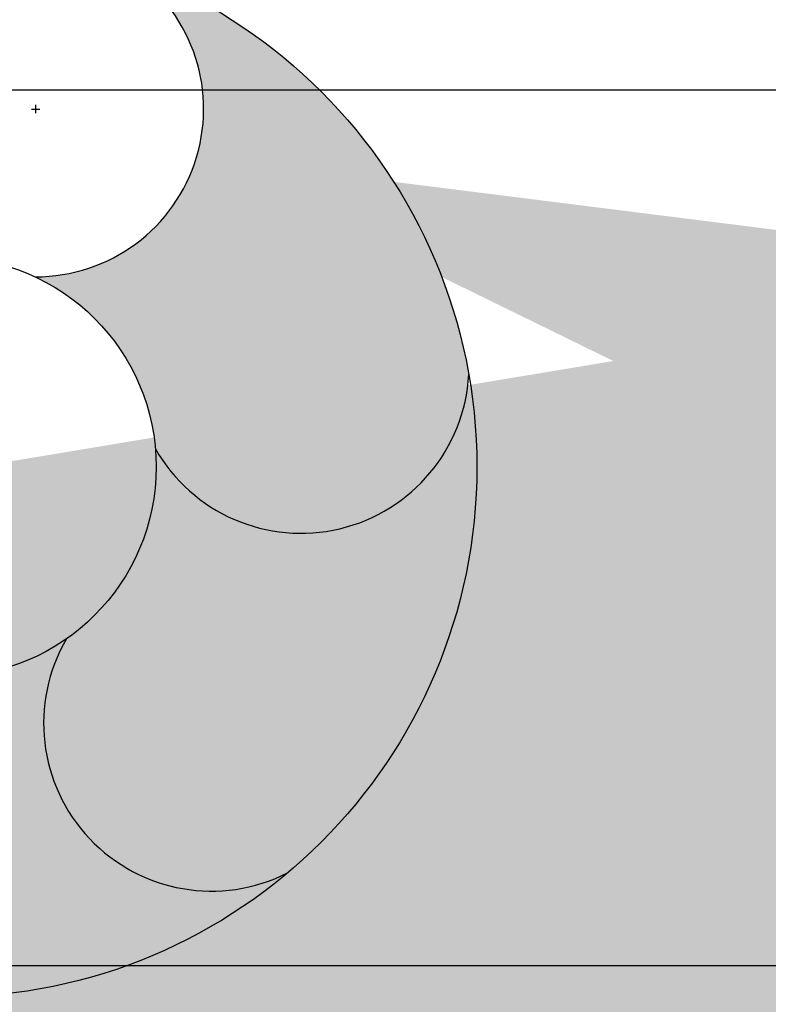
# Model space of a CAD drawing. Units: millimetres. Extents: x -22994 to 29398, y -19990 to 20176.
# Tile 117 of 135: x 229 to 245, y 135 to 156. Entities that reach past the tile are written whole.
import ezdxf

# ---------------------------------------------------------------- set-up
doc = ezdxf.new("R2010")
doc.units = ezdxf.units.MM
doc.header["$MEASUREMENT"] = 0
for name, color, linetype, lineweight in [('M-DIMS', 2, 'Continuous', 18), ('M-EQPM', 7, 'Continuous', 25), ('M-EQPM-PATT', 7, 'Continuous', 18)]:
    doc.layers.add(name, color=color, linetype=linetype, lineweight=lineweight)
doc.styles.get("Standard").update_dxf_attribs({"font": 'arial.ttf'})
doc.dimstyles.get("Standard").update_dxf_attribs({"dimtxt": 0.18, "dimasz": 10000, "dimexe": 0.18, "dimexo": 0.0625, "dimgap": 0.09, "dimtad": 0, "dimtih": 1, "dimtoh": 1, "dimdec": 0, "dimzin": 0, "dimdsep": 46, "dimtxsty": 'Standard', "dimcen": 0.09, "dimadec": 0, "dimazin": 0, "dimtfac": 1, "dimtdec": 0, "dimtofl": 0, "dimtmove": 0, "dimatfit": 3, "dimfxl": 1, "dimtolj": 1, "dimtzin": 0, "dimlwd": 30, "dimarcsym": 0})

# ---------------------------------------------------------------- blocks, each defined once
blk = doc.blocks.new('*D2')
at = {"layer": 'Defpoints', "color": 0, "transparency": 16777216}
for p in [(6.677, 10.271), (290.852, 10.271), (290.852, -5.079)]:
    blk.add_point(p, dxfattribs=at)
at = {"layer": 'M-DIMS', "color": 0, "lineweight": -2, "transparency": 16777216}
for p, q in [((6.677, 10.209), (6.677, -5.259)), ((290.852, 10.209), (290.852, -5.259))]:
    blk.add_line(p, q, dxfattribs=at)
at = {"layer": 'M-DIMS', "color": 0, "lineweight": 30, "transparency": 16777216}
for p, q in [((-9993.323, -5.079), (-19993.323, -5.079)), ((10290.852, -5.079), (20290.852, -5.079))]:
    blk.add_line(p, q, dxfattribs=at)
at = {"layer": 'M-DIMS', "color": 0, "transparency": 16777216}
for points in [[(-9993.323, 1661.588), (-9993.323, -1671.745), (6.677, -5.079)], [(10290.852, 1661.588), (10290.852, -1671.745), (290.852, -5.079)]]:
    blk.add_solid(points, dxfattribs=at)
at = {"layer": 'M-DIMS', "color": 0, "transparency": 16777216, "insert": (148.765, -5.079), "char_height": 0.18, "attachment_point": 5}
blk.add_mtext('\\A1;284.2', dxfattribs=at)
blk = doc.blocks.new('*D3')
at = {"layer": 'Defpoints', "color": 0, "transparency": 16777216}
for p in [(110.265, 204.165), (110.265, 176.366), (95.833, 127.967)]:
    blk.add_point(p, dxfattribs=at)
at = {"layer": 'M-DIMS', "color": 0, "lineweight": -2, "transparency": 16777216}
for p, q in [((95.833, 128.03), (95.833, 204.345)), ((110.265, 176.429), (110.265, 204.345))]:
    blk.add_line(p, q, dxfattribs=at)
at = {"layer": 'M-DIMS', "color": 0, "lineweight": 30, "transparency": 16777216}
for p, q in [((-9904.167, 204.165), (-19904.167, 204.165)), ((10110.265, 204.165), (20110.265, 204.165))]:
    blk.add_line(p, q, dxfattribs=at)
at = {"layer": 'M-DIMS', "color": 0, "transparency": 16777216}
for points in [[(-9904.167, 1870.832), (-9904.167, -1462.501), (95.833, 204.165)], [(10110.265, 1870.832), (10110.265, -1462.501), (110.265, 204.165)]]:
    blk.add_solid(points, dxfattribs=at)
at = {"layer": 'M-DIMS', "color": 0, "transparency": 16777216, "insert": (103.049, 204.165), "char_height": 0.18, "attachment_point": 5}
blk.add_mtext('\\A1;14.432', dxfattribs=at)
blk = doc.blocks.new('*D4')
at = {"layer": 'Defpoints', "color": 0, "transparency": 16777216}
for p in [(116.265, 204.165), (110.265, 176.366), (116.265, 176.366)]:
    blk.add_point(p, dxfattribs=at)
at = {"layer": 'M-DIMS', "color": 0, "lineweight": -2, "transparency": 16777216}
for p, q in [((110.265, 176.429), (110.265, 204.345)), ((116.265, 176.429), (116.265, 204.345))]:
    blk.add_line(p, q, dxfattribs=at)
at = {"layer": 'M-DIMS', "color": 0, "lineweight": 30, "transparency": 16777216}
for p, q in [((-9889.735, 204.165), (-19889.735, 204.165)), ((10116.265, 204.165), (20116.265, 204.165))]:
    blk.add_line(p, q, dxfattribs=at)
at = {"layer": 'M-DIMS', "color": 0, "transparency": 16777216}
for points in [[(-9889.735, 1870.832), (-9889.735, -1462.501), (110.265, 204.165)], [(10116.265, 1870.832), (10116.265, -1462.501), (116.265, 204.165)]]:
    blk.add_solid(points, dxfattribs=at)
at = {"layer": 'M-DIMS', "color": 0, "transparency": 16777216, "insert": (113.265, 204.165), "char_height": 0.18, "attachment_point": 5}
blk.add_mtext('\\A1;6', dxfattribs=at)
blk = doc.blocks.new('*D5')
at = {"layer": 'Defpoints', "color": 0, "transparency": 16777216}
for p in [(181.265, 204.165), (116.265, 176.366), (181.265, 176.366)]:
    blk.add_point(p, dxfattribs=at)
at = {"layer": 'M-DIMS', "color": 0, "lineweight": -2, "transparency": 16777216}
for p, q in [((116.265, 176.429), (116.265, 204.345)), ((181.265, 176.429), (181.265, 204.345))]:
    blk.add_line(p, q, dxfattribs=at)
at = {"layer": 'M-DIMS', "color": 0, "lineweight": 30, "transparency": 16777216}
for p, q in [((-9883.735, 204.165), (-19883.735, 204.165)), ((10181.265, 204.165), (20181.265, 204.165))]:
    blk.add_line(p, q, dxfattribs=at)
at = {"layer": 'M-DIMS', "color": 0, "transparency": 16777216}
for points in [[(-9883.735, 1870.832), (-9883.735, -1462.501), (116.265, 204.165)], [(10181.265, 1870.832), (10181.265, -1462.501), (181.265, 204.165)]]:
    blk.add_solid(points, dxfattribs=at)
at = {"layer": 'M-DIMS', "color": 0, "transparency": 16777216, "insert": (148.765, 204.165), "char_height": 0.18, "attachment_point": 5}
blk.add_mtext('\\A1;65', dxfattribs=at)
blk = doc.blocks.new('*D6')
at = {"layer": 'Defpoints', "color": 0, "transparency": 16777216}
for p in [(187.265, 204.165), (181.265, 176.366), (187.265, 176.366)]:
    blk.add_point(p, dxfattribs=at)
at = {"layer": 'M-DIMS', "color": 0, "lineweight": -2, "transparency": 16777216}
for p, q in [((181.265, 176.429), (181.265, 204.345)), ((187.265, 176.429), (187.265, 204.345))]:
    blk.add_line(p, q, dxfattribs=at)
at = {"layer": 'M-DIMS', "color": 0, "lineweight": 30, "transparency": 16777216}
for p, q in [((-9818.735, 204.165), (-19818.735, 204.165)), ((10187.265, 204.165), (20187.265, 204.165))]:
    blk.add_line(p, q, dxfattribs=at)
at = {"layer": 'M-DIMS', "color": 0, "transparency": 16777216}
for points in [[(-9818.735, 1870.832), (-9818.735, -1462.501), (181.265, 204.165)], [(10187.265, 1870.832), (10187.265, -1462.501), (187.265, 204.165)]]:
    blk.add_solid(points, dxfattribs=at)
at = {"layer": 'M-DIMS', "color": 0, "transparency": 16777216, "insert": (184.265, 204.165), "char_height": 0.18, "attachment_point": 5}
blk.add_mtext('\\A1;6', dxfattribs=at)
blk = doc.blocks.new('*D7')
at = {"layer": 'Defpoints', "color": 0, "transparency": 16777216}
for p in [(201.697, 204.165), (187.265, 176.366), (201.697, 127.967)]:
    blk.add_point(p, dxfattribs=at)
at = {"layer": 'M-DIMS', "color": 0, "lineweight": -2, "transparency": 16777216}
for p, q in [((187.265, 176.429), (187.265, 204.345)), ((201.697, 128.03), (201.697, 204.345))]:
    blk.add_line(p, q, dxfattribs=at)
at = {"layer": 'M-DIMS', "color": 0, "lineweight": 30, "transparency": 16777216}
for p, q in [((-9812.735, 204.165), (-19812.735, 204.165)), ((10201.697, 204.165), (20201.697, 204.165))]:
    blk.add_line(p, q, dxfattribs=at)
at = {"layer": 'M-DIMS', "color": 0, "transparency": 16777216}
for points in [[(-9812.735, 1870.832), (-9812.735, -1462.501), (187.265, 204.165)], [(10201.697, 1870.832), (10201.697, -1462.501), (201.697, 204.165)]]:
    blk.add_solid(points, dxfattribs=at)
at = {"layer": 'M-DIMS', "color": 0, "transparency": 16777216, "insert": (194.481, 204.165), "char_height": 0.18, "attachment_point": 5}
blk.add_mtext('\\A1;14.432', dxfattribs=at)
blk = doc.blocks.new('*D8')
at = {"layer": 'Defpoints', "color": 0, "transparency": 16777216}
for p in [(227.648, 204.165), (227.648, 146.73), (201.697, 127.967)]:
    blk.add_point(p, dxfattribs=at)
at = {"layer": 'M-DIMS', "color": 0, "lineweight": -2, "transparency": 16777216}
for p, q in [((201.697, 128.03), (201.697, 204.345)), ((227.648, 146.792), (227.648, 204.345))]:
    blk.add_line(p, q, dxfattribs=at)
at = {"layer": 'M-DIMS', "color": 0, "lineweight": 30, "transparency": 16777216}
for p, q in [((-9798.303, 204.165), (-19798.303, 204.165)), ((10227.648, 204.165), (20227.648, 204.165))]:
    blk.add_line(p, q, dxfattribs=at)
at = {"layer": 'M-DIMS', "color": 0, "transparency": 16777216}
for points in [[(-9798.303, 1870.832), (-9798.303, -1462.501), (201.697, 204.165)], [(10227.648, 1870.832), (10227.648, -1462.501), (227.648, 204.165)]]:
    blk.add_solid(points, dxfattribs=at)
at = {"layer": 'M-DIMS', "color": 0, "transparency": 16777216, "insert": (214.673, 204.165), "char_height": 0.18, "attachment_point": 5}
blk.add_mtext('\\A1;25.95', dxfattribs=at)
blk = doc.blocks.new('*D9')
at = {"layer": 'Defpoints', "color": 0, "transparency": 16777216}
for p in [(187.265, 176.366), (306.202, 176.366), (290.852, 10.271)]:
    blk.add_point(p, dxfattribs=at)
at = {"layer": 'M-DIMS', "color": 0, "lineweight": 30, "transparency": 16777216}
for p, q in [((306.202, 10176.366), (306.202, 20176.366)), ((306.202, -9989.729), (306.202, -19989.729))]:
    blk.add_line(p, q, dxfattribs=at)
at = {"layer": 'M-DIMS', "color": 0, "lineweight": -2, "transparency": 16777216}
for p, q in [((187.327, 176.366), (306.382, 176.366)), ((290.915, 10.271), (306.382, 10.271))]:
    blk.add_line(p, q, dxfattribs=at)
at = {"layer": 'M-DIMS', "color": 0, "transparency": 16777216}
for points in [[(-1360.465, 10176.366), (1972.869, 10176.366), (306.202, 176.366)], [(-1360.465, -9989.729), (1972.869, -9989.729), (306.202, 10.271)]]:
    blk.add_solid(points, dxfattribs=at)
at = {"layer": 'M-DIMS', "color": 0, "transparency": 16777216, "insert": (306.202, 93.319), "char_height": 0.18, "attachment_point": 5}
blk.add_mtext('\\A1;166.1', dxfattribs=at)
blk = doc.blocks.new('*D10')
at = {"layer": 'Defpoints', "color": 0, "transparency": 16777216}
for p in [(125.65, 136.071), (133.346, 136.071), (133.346, -5.079)]:
    blk.add_point(p, dxfattribs=at)
at = {"layer": 'M-DIMS', "color": 0, "lineweight": -2, "transparency": 16777216}
for p, q in [((125.65, 136.009), (125.65, -5.259)), ((133.346, 136.009), (133.346, -5.259))]:
    blk.add_line(p, q, dxfattribs=at)
at = {"layer": 'M-DIMS', "color": 0, "lineweight": 30, "transparency": 16777216}
for p, q in [((-9874.35, -5.079), (-19874.35, -5.079)), ((10133.346, -5.079), (20133.346, -5.079))]:
    blk.add_line(p, q, dxfattribs=at)
at = {"layer": 'M-DIMS', "color": 0, "transparency": 16777216}
for points in [[(-9874.35, 1661.588), (-9874.35, -1671.745), (125.65, -5.079)], [(10133.346, 1661.588), (10133.346, -1671.745), (133.346, -5.079)]]:
    blk.add_solid(points, dxfattribs=at)
at = {"layer": 'M-DIMS', "color": 0, "transparency": 16777216, "insert": (129.498, -5.079), "char_height": 0.18, "attachment_point": 5}
blk.add_mtext('\\A1;7.696', dxfattribs=at)
blk = doc.blocks.new('*D11')
at = {"layer": 'Defpoints', "color": 0, "transparency": 16777216}
for p in [(133.346, 136.071), (135.65, 136.071), (135.65, -5.079)]:
    blk.add_point(p, dxfattribs=at)
at = {"layer": 'M-DIMS', "color": 0, "lineweight": -2, "transparency": 16777216}
for p, q in [((133.346, 136.009), (133.346, -5.259)), ((135.65, 136.009), (135.65, -5.259))]:
    blk.add_line(p, q, dxfattribs=at)
at = {"layer": 'M-DIMS', "color": 0, "lineweight": 30, "transparency": 16777216}
for p, q in [((-9866.654, -5.079), (-19866.654, -5.079)), ((10135.65, -5.079), (20135.65, -5.079))]:
    blk.add_line(p, q, dxfattribs=at)
at = {"layer": 'M-DIMS', "color": 0, "transparency": 16777216}
for points in [[(-9866.654, 1661.588), (-9866.654, -1671.745), (133.346, -5.079)], [(10135.65, 1661.588), (10135.65, -1671.745), (135.65, -5.079)]]:
    blk.add_solid(points, dxfattribs=at)
at = {"layer": 'M-DIMS', "color": 0, "transparency": 16777216, "insert": (134.498, -5.079), "char_height": 0.18, "attachment_point": 5}
blk.add_mtext('\\A1;2.304', dxfattribs=at)
blk = doc.blocks.new('*D12')
at = {"layer": 'Defpoints', "color": 0, "transparency": 16777216}
for p in [(135.65, 136.071), (145.65, 136.071), (145.65, -5.079)]:
    blk.add_point(p, dxfattribs=at)
at = {"layer": 'M-DIMS', "color": 0, "lineweight": -2, "transparency": 16777216}
for p, q in [((135.65, 136.009), (135.65, -5.259)), ((145.65, 136.009), (145.65, -5.259))]:
    blk.add_line(p, q, dxfattribs=at)
at = {"layer": 'M-DIMS', "color": 0, "lineweight": 30, "transparency": 16777216}
for p, q in [((-9864.35, -5.079), (-19864.35, -5.079)), ((10145.65, -5.079), (20145.65, -5.079))]:
    blk.add_line(p, q, dxfattribs=at)
at = {"layer": 'M-DIMS', "color": 0, "transparency": 16777216}
for points in [[(-9864.35, 1661.588), (-9864.35, -1671.745), (135.65, -5.079)], [(10145.65, 1661.588), (10145.65, -1671.745), (145.65, -5.079)]]:
    blk.add_solid(points, dxfattribs=at)
at = {"layer": 'M-DIMS', "color": 0, "transparency": 16777216, "insert": (140.65, -5.079), "char_height": 0.18, "attachment_point": 5}
blk.add_mtext('\\A1;10', dxfattribs=at)
blk = doc.blocks.new('*D13')
at = {"layer": 'Defpoints', "color": 0, "transparency": 16777216}
for p in [(145.65, 136.071), (155.65, 136.071), (155.65, -5.079)]:
    blk.add_point(p, dxfattribs=at)
at = {"layer": 'M-DIMS', "color": 0, "lineweight": -2, "transparency": 16777216}
for p, q in [((145.65, 136.009), (145.65, -5.259)), ((155.65, 136.009), (155.65, -5.259))]:
    blk.add_line(p, q, dxfattribs=at)
at = {"layer": 'M-DIMS', "color": 0, "lineweight": 30, "transparency": 16777216}
for p, q in [((-9854.35, -5.079), (-19854.35, -5.079)), ((10155.65, -5.079), (20155.65, -5.079))]:
    blk.add_line(p, q, dxfattribs=at)
at = {"layer": 'M-DIMS', "color": 0, "transparency": 16777216}
for points in [[(-9854.35, 1661.588), (-9854.35, -1671.745), (145.65, -5.079)], [(10155.65, 1661.588), (10155.65, -1671.745), (155.65, -5.079)]]:
    blk.add_solid(points, dxfattribs=at)
at = {"layer": 'M-DIMS', "color": 0, "transparency": 16777216, "insert": (150.65, -5.079), "char_height": 0.18, "attachment_point": 5}
blk.add_mtext('\\A1;10', dxfattribs=at)
blk = doc.blocks.new('*D14')
at = {"layer": 'Defpoints', "color": 0, "transparency": 16777216}
for p in [(155.65, 136.071), (165.65, 136.071), (165.65, -5.079)]:
    blk.add_point(p, dxfattribs=at)
at = {"layer": 'M-DIMS', "color": 0, "lineweight": -2, "transparency": 16777216}
for p, q in [((155.65, 136.009), (155.65, -5.259)), ((165.65, 136.009), (165.65, -5.259))]:
    blk.add_line(p, q, dxfattribs=at)
at = {"layer": 'M-DIMS', "color": 0, "lineweight": 30, "transparency": 16777216}
for p, q in [((-9844.35, -5.079), (-19844.35, -5.079)), ((10165.65, -5.079), (20165.65, -5.079))]:
    blk.add_line(p, q, dxfattribs=at)
at = {"layer": 'M-DIMS', "color": 0, "transparency": 16777216}
for points in [[(-9844.35, 1661.588), (-9844.35, -1671.745), (155.65, -5.079)], [(10165.65, 1661.588), (10165.65, -1671.745), (165.65, -5.079)]]:
    blk.add_solid(points, dxfattribs=at)
at = {"layer": 'M-DIMS', "color": 0, "transparency": 16777216, "insert": (160.65, -5.079), "char_height": 0.18, "attachment_point": 5}
blk.add_mtext('\\A1;10', dxfattribs=at)
blk = doc.blocks.new('*D15')
at = {"layer": 'Defpoints', "color": 0, "transparency": 16777216}
for p in [(173.346, 154.788), (173.346, 136.071), (306.202, 136.071)]:
    blk.add_point(p, dxfattribs=at)
at = {"layer": 'M-DIMS', "color": 0, "lineweight": 30, "transparency": 16777216}
for p, q in [((306.202, 10154.788), (306.202, 20154.788)), ((306.202, -9863.929), (306.202, -19863.929))]:
    blk.add_line(p, q, dxfattribs=at)
at = {"layer": 'M-DIMS', "color": 0, "lineweight": -2, "transparency": 16777216}
for p, q in [((173.408, 154.788), (306.382, 154.788)), ((173.408, 136.071), (306.382, 136.071))]:
    blk.add_line(p, q, dxfattribs=at)
at = {"layer": 'M-DIMS', "color": 0, "transparency": 16777216}
for points in [[(-1360.465, 10154.788), (1972.869, 10154.788), (306.202, 154.788)], [(-1360.465, -9863.929), (1972.869, -9863.929), (306.202, 136.071)]]:
    blk.add_solid(points, dxfattribs=at)
at = {"layer": 'M-DIMS', "color": 0, "transparency": 16777216, "insert": (306.202, 145.43), "char_height": 0.18, "attachment_point": 5}
blk.add_mtext('\\A1;18.717', dxfattribs=at)
blk = doc.blocks.new('*D16')
at = {"layer": 'Defpoints', "color": 0, "transparency": 16777216}
for p in [(120.17, 204.165), (110.466, 48.035), (120.17, 48.035)]:
    blk.add_point(p, dxfattribs=at)
at = {"layer": 'M-DIMS', "color": 0, "lineweight": -2, "transparency": 16777216}
for p, q in [((110.466, 48.097), (110.466, 204.345)), ((120.17, 48.097), (120.17, 204.345))]:
    blk.add_line(p, q, dxfattribs=at)
at = {"layer": 'M-DIMS', "color": 0, "lineweight": 30, "transparency": 16777216}
for p, q in [((-9889.534, 204.165), (-19889.534, 204.165)), ((10120.17, 204.165), (20120.17, 204.165))]:
    blk.add_line(p, q, dxfattribs=at)
at = {"layer": 'M-DIMS', "color": 0, "transparency": 16777216}
for points in [[(-9889.534, 1870.832), (-9889.534, -1462.501), (110.466, 204.165)], [(10120.17, 1870.832), (10120.17, -1462.501), (120.17, 204.165)]]:
    blk.add_solid(points, dxfattribs=at)
at = {"layer": 'M-DIMS', "color": 0, "transparency": 16777216, "insert": (115.318, 204.165), "char_height": 0.18, "attachment_point": 5}
blk.add_mtext('\\A1;9.704', dxfattribs=at)
blk = doc.blocks.new('*D17')
at = {"layer": 'Defpoints', "color": 0, "transparency": 16777216}
for p in [(126.17, 204.165), (120.17, 48.035), (126.17, 48.035)]:
    blk.add_point(p, dxfattribs=at)
at = {"layer": 'M-DIMS', "color": 0, "lineweight": -2, "transparency": 16777216}
for p, q in [((120.17, 48.097), (120.17, 204.345)), ((126.17, 48.097), (126.17, 204.345))]:
    blk.add_line(p, q, dxfattribs=at)
at = {"layer": 'M-DIMS', "color": 0, "lineweight": 30, "transparency": 16777216}
for p, q in [((-9879.83, 204.165), (-19879.83, 204.165)), ((10126.17, 204.165), (20126.17, 204.165))]:
    blk.add_line(p, q, dxfattribs=at)
at = {"layer": 'M-DIMS', "color": 0, "transparency": 16777216}
for points in [[(-9879.83, 1870.832), (-9879.83, -1462.501), (120.17, 204.165)], [(10126.17, 1870.832), (10126.17, -1462.501), (126.17, 204.165)]]:
    blk.add_solid(points, dxfattribs=at)
at = {"layer": 'M-DIMS', "color": 0, "transparency": 16777216, "insert": (123.17, 204.165), "char_height": 0.18, "attachment_point": 5}
blk.add_mtext('\\A1;6', dxfattribs=at)
blk = doc.blocks.new('*D18')
at = {"layer": 'Defpoints', "color": 0, "transparency": 16777216}
for p in [(132.17, 204.165), (126.17, 48.035), (132.17, 48.035)]:
    blk.add_point(p, dxfattribs=at)
at = {"layer": 'M-DIMS', "color": 0, "lineweight": -2, "transparency": 16777216}
for p, q in [((126.17, 48.097), (126.17, 204.345)), ((132.17, 48.097), (132.17, 204.345))]:
    blk.add_line(p, q, dxfattribs=at)
at = {"layer": 'M-DIMS', "color": 0, "lineweight": 30, "transparency": 16777216}
for p, q in [((-9873.83, 204.165), (-19873.83, 204.165)), ((10132.17, 204.165), (20132.17, 204.165))]:
    blk.add_line(p, q, dxfattribs=at)
at = {"layer": 'M-DIMS', "color": 0, "transparency": 16777216}
for points in [[(-9873.83, 1870.832), (-9873.83, -1462.501), (126.17, 204.165)], [(10132.17, 1870.832), (10132.17, -1462.501), (132.17, 204.165)]]:
    blk.add_solid(points, dxfattribs=at)
at = {"layer": 'M-DIMS', "color": 0, "transparency": 16777216, "insert": (129.17, 204.165), "char_height": 0.18, "attachment_point": 5}
blk.add_mtext('\\A1;6', dxfattribs=at)
blk = doc.blocks.new('*D19')
at = {"layer": 'Defpoints', "color": 0, "transparency": 16777216}
for p in [(138.17, 204.165), (132.17, 48.035), (138.17, 48.035)]:
    blk.add_point(p, dxfattribs=at)
at = {"layer": 'M-DIMS', "color": 0, "lineweight": -2, "transparency": 16777216}
for p, q in [((132.17, 48.097), (132.17, 204.345)), ((138.17, 48.097), (138.17, 204.345))]:
    blk.add_line(p, q, dxfattribs=at)
at = {"layer": 'M-DIMS', "color": 0, "lineweight": 30, "transparency": 16777216}
for p, q in [((-9867.83, 204.165), (-19867.83, 204.165)), ((10138.17, 204.165), (20138.17, 204.165))]:
    blk.add_line(p, q, dxfattribs=at)
at = {"layer": 'M-DIMS', "color": 0, "transparency": 16777216}
for points in [[(-9867.83, 1870.832), (-9867.83, -1462.501), (132.17, 204.165)], [(10138.17, 1870.832), (10138.17, -1462.501), (138.17, 204.165)]]:
    blk.add_solid(points, dxfattribs=at)
at = {"layer": 'M-DIMS', "color": 0, "transparency": 16777216, "insert": (135.17, 204.165), "char_height": 0.18, "attachment_point": 5}
blk.add_mtext('\\A1;6', dxfattribs=at)
blk = doc.blocks.new('*D20')
at = {"layer": 'Defpoints', "color": 0, "transparency": 16777216}
for p in [(144.17, 204.165), (138.17, 48.035), (144.17, 48.035)]:
    blk.add_point(p, dxfattribs=at)
at = {"layer": 'M-DIMS', "color": 0, "lineweight": -2, "transparency": 16777216}
for p, q in [((138.17, 48.097), (138.17, 204.345)), ((144.17, 48.097), (144.17, 204.345))]:
    blk.add_line(p, q, dxfattribs=at)
at = {"layer": 'M-DIMS', "color": 0, "lineweight": 30, "transparency": 16777216}
for p, q in [((-9861.83, 204.165), (-19861.83, 204.165)), ((10144.17, 204.165), (20144.17, 204.165))]:
    blk.add_line(p, q, dxfattribs=at)
at = {"layer": 'M-DIMS', "color": 0, "transparency": 16777216}
for points in [[(-9861.83, 1870.832), (-9861.83, -1462.501), (138.17, 204.165)], [(10144.17, 1870.832), (10144.17, -1462.501), (144.17, 204.165)]]:
    blk.add_solid(points, dxfattribs=at)
at = {"layer": 'M-DIMS', "color": 0, "transparency": 16777216, "insert": (141.17, 204.165), "char_height": 0.18, "attachment_point": 5}
blk.add_mtext('\\A1;6', dxfattribs=at)
blk = doc.blocks.new('*D21')
at = {"layer": 'Defpoints', "color": 0, "transparency": 16777216}
for p in [(149.116, 204.165), (144.17, 48.035), (149.116, 48.035)]:
    blk.add_point(p, dxfattribs=at)
at = {"layer": 'M-DIMS', "color": 0, "lineweight": -2, "transparency": 16777216}
for p, q in [((144.17, 48.097), (144.17, 204.345)), ((149.116, 48.097), (149.116, 204.345))]:
    blk.add_line(p, q, dxfattribs=at)
at = {"layer": 'M-DIMS', "color": 0, "lineweight": 30, "transparency": 16777216}
for p, q in [((-9855.83, 204.165), (-19855.83, 204.165)), ((10149.116, 204.165), (20149.116, 204.165))]:
    blk.add_line(p, q, dxfattribs=at)
at = {"layer": 'M-DIMS', "color": 0, "transparency": 16777216}
for points in [[(-9855.83, 1870.832), (-9855.83, -1462.501), (144.17, 204.165)], [(10149.116, 1870.832), (10149.116, -1462.501), (149.116, 204.165)]]:
    blk.add_solid(points, dxfattribs=at)
at = {"layer": 'M-DIMS', "color": 0, "transparency": 16777216, "insert": (146.643, 204.165), "char_height": 0.18, "attachment_point": 5}
blk.add_mtext('\\A1;4.945', dxfattribs=at)
blk = doc.blocks.new('*D22')
at = {"layer": 'Defpoints', "color": 0, "transparency": 16777216}
for p in [(149.116, 30.99), (155.116, 30.99), (155.116, -5.079)]:
    blk.add_point(p, dxfattribs=at)
at = {"layer": 'M-DIMS', "color": 0, "lineweight": -2, "transparency": 16777216}
for p, q in [((149.116, 30.927), (149.116, -5.259)), ((155.116, 30.927), (155.116, -5.259))]:
    blk.add_line(p, q, dxfattribs=at)
at = {"layer": 'M-DIMS', "color": 0, "lineweight": 30, "transparency": 16777216}
for p, q in [((-9850.884, -5.079), (-19850.884, -5.079)), ((10155.116, -5.079), (20155.116, -5.079))]:
    blk.add_line(p, q, dxfattribs=at)
at = {"layer": 'M-DIMS', "color": 0, "transparency": 16777216}
for points in [[(-9850.884, 1661.588), (-9850.884, -1671.745), (149.116, -5.079)], [(10155.116, 1661.588), (10155.116, -1671.745), (155.116, -5.079)]]:
    blk.add_solid(points, dxfattribs=at)
at = {"layer": 'M-DIMS', "color": 0, "transparency": 16777216, "insert": (152.116, -5.079), "char_height": 0.18, "attachment_point": 5}
blk.add_mtext('\\A1;6', dxfattribs=at)
blk = doc.blocks.new('*D23')
at = {"layer": 'Defpoints', "color": 0, "transparency": 16777216}
for p in [(155.116, 30.99), (161.116, 30.99), (161.116, -5.079)]:
    blk.add_point(p, dxfattribs=at)
at = {"layer": 'M-DIMS', "color": 0, "lineweight": -2, "transparency": 16777216}
for p, q in [((155.116, 30.927), (155.116, -5.259)), ((161.116, 30.927), (161.116, -5.259))]:
    blk.add_line(p, q, dxfattribs=at)
at = {"layer": 'M-DIMS', "color": 0, "lineweight": 30, "transparency": 16777216}
for p, q in [((-9844.884, -5.079), (-19844.884, -5.079)), ((10161.116, -5.079), (20161.116, -5.079))]:
    blk.add_line(p, q, dxfattribs=at)
at = {"layer": 'M-DIMS', "color": 0, "transparency": 16777216}
for points in [[(-9844.884, 1661.588), (-9844.884, -1671.745), (155.116, -5.079)], [(10161.116, 1661.588), (10161.116, -1671.745), (161.116, -5.079)]]:
    blk.add_solid(points, dxfattribs=at)
at = {"layer": 'M-DIMS', "color": 0, "transparency": 16777216, "insert": (158.116, -5.079), "char_height": 0.18, "attachment_point": 5}
blk.add_mtext('\\A1;6', dxfattribs=at)
blk = doc.blocks.new('*D24')
at = {"layer": 'Defpoints', "color": 0, "transparency": 16777216}
for p in [(161.116, 30.99), (166.439, 30.99), (166.439, -5.079)]:
    blk.add_point(p, dxfattribs=at)
at = {"layer": 'M-DIMS', "color": 0, "lineweight": -2, "transparency": 16777216}
for p, q in [((161.116, 30.927), (161.116, -5.259)), ((166.439, 30.927), (166.439, -5.259))]:
    blk.add_line(p, q, dxfattribs=at)
at = {"layer": 'M-DIMS', "color": 0, "lineweight": 30, "transparency": 16777216}
for p, q in [((-9838.884, -5.079), (-19838.884, -5.079)), ((10166.439, -5.079), (20166.439, -5.079))]:
    blk.add_line(p, q, dxfattribs=at)
at = {"layer": 'M-DIMS', "color": 0, "transparency": 16777216}
for points in [[(-9838.884, 1661.588), (-9838.884, -1671.745), (161.116, -5.079)], [(10166.439, 1661.588), (10166.439, -1671.745), (166.439, -5.079)]]:
    blk.add_solid(points, dxfattribs=at)
at = {"layer": 'M-DIMS', "color": 0, "transparency": 16777216, "insert": (163.777, -5.079), "char_height": 0.18, "attachment_point": 5}
blk.add_mtext('\\A1;5.323', dxfattribs=at)
blk = doc.blocks.new('*D25')
at = {"layer": 'Defpoints', "color": 0, "transparency": 16777216}
for p in [(166.439, 30.99), (172.439, 30.99), (172.439, -5.079)]:
    blk.add_point(p, dxfattribs=at)
at = {"layer": 'M-DIMS', "color": 0, "lineweight": -2, "transparency": 16777216}
for p, q in [((166.439, 30.927), (166.439, -5.259)), ((172.439, 30.927), (172.439, -5.259))]:
    blk.add_line(p, q, dxfattribs=at)
at = {"layer": 'M-DIMS', "color": 0, "lineweight": 30, "transparency": 16777216}
for p, q in [((-9833.561, -5.079), (-19833.561, -5.079)), ((10172.439, -5.079), (20172.439, -5.079))]:
    blk.add_line(p, q, dxfattribs=at)
at = {"layer": 'M-DIMS', "color": 0, "transparency": 16777216}
for points in [[(-9833.561, 1661.588), (-9833.561, -1671.745), (166.439, -5.079)], [(10172.439, 1661.588), (10172.439, -1671.745), (172.439, -5.079)]]:
    blk.add_solid(points, dxfattribs=at)
at = {"layer": 'M-DIMS', "color": 0, "transparency": 16777216, "insert": (169.439, -5.079), "char_height": 0.18, "attachment_point": 5}
blk.add_mtext('\\A1;6', dxfattribs=at)
blk = doc.blocks.new('*D26')
at = {"layer": 'Defpoints', "color": 0, "transparency": 16777216}
for p in [(172.439, 30.99), (178.439, 30.99), (178.439, -5.079)]:
    blk.add_point(p, dxfattribs=at)
at = {"layer": 'M-DIMS', "color": 0, "lineweight": -2, "transparency": 16777216}
for p, q in [((172.439, 30.927), (172.439, -5.259)), ((178.439, 30.927), (178.439, -5.259))]:
    blk.add_line(p, q, dxfattribs=at)
at = {"layer": 'M-DIMS', "color": 0, "lineweight": 30, "transparency": 16777216}
for p, q in [((-9827.561, -5.079), (-19827.561, -5.079)), ((10178.439, -5.079), (20178.439, -5.079))]:
    blk.add_line(p, q, dxfattribs=at)
at = {"layer": 'M-DIMS', "color": 0, "transparency": 16777216}
for points in [[(-9827.561, 1661.588), (-9827.561, -1671.745), (172.439, -5.079)], [(10178.439, 1661.588), (10178.439, -1671.745), (178.439, -5.079)]]:
    blk.add_solid(points, dxfattribs=at)
at = {"layer": 'M-DIMS', "color": 0, "transparency": 16777216, "insert": (175.439, -5.079), "char_height": 0.18, "attachment_point": 5}
blk.add_mtext('\\A1;6', dxfattribs=at)
blk = doc.blocks.new('*D27')
at = {"layer": 'Defpoints', "color": 0, "transparency": 16777216}
for p in [(178.439, 30.99), (188.117, 30.99), (188.117, -5.079)]:
    blk.add_point(p, dxfattribs=at)
at = {"layer": 'M-DIMS', "color": 0, "lineweight": -2, "transparency": 16777216}
for p, q in [((178.439, 30.927), (178.439, -5.259)), ((188.117, 30.927), (188.117, -5.259))]:
    blk.add_line(p, q, dxfattribs=at)
at = {"layer": 'M-DIMS', "color": 0, "lineweight": 30, "transparency": 16777216}
for p, q in [((-9821.561, -5.079), (-19821.561, -5.079)), ((10188.117, -5.079), (20188.117, -5.079))]:
    blk.add_line(p, q, dxfattribs=at)
at = {"layer": 'M-DIMS', "color": 0, "transparency": 16777216}
for points in [[(-9821.561, 1661.588), (-9821.561, -1671.745), (178.439, -5.079)], [(10188.117, 1661.588), (10188.117, -1671.745), (188.117, -5.079)]]:
    blk.add_solid(points, dxfattribs=at)
at = {"layer": 'M-DIMS', "color": 0, "transparency": 16777216, "insert": (183.278, -5.079), "char_height": 0.18, "attachment_point": 5}
blk.add_mtext('\\A1;9.679', dxfattribs=at)
blk = doc.blocks.new('*D28')
at = {"layer": 'Defpoints', "color": 0, "transparency": 16777216}
for p in [(188.117, 48.035), (306.202, 48.035), (188.117, 30.99)]:
    blk.add_point(p, dxfattribs=at)
at = {"layer": 'M-DIMS', "color": 0, "lineweight": 30, "transparency": 16777216}
for p, q in [((306.202, 10048.035), (306.202, 20048.035)), ((306.202, -9969.01), (306.202, -19969.01))]:
    blk.add_line(p, q, dxfattribs=at)
at = {"layer": 'M-DIMS', "color": 0, "lineweight": -2, "transparency": 16777216}
for p, q in [((188.18, 48.035), (306.382, 48.035)), ((188.18, 30.99), (306.382, 30.99))]:
    blk.add_line(p, q, dxfattribs=at)
at = {"layer": 'M-DIMS', "color": 0, "transparency": 16777216}
for points in [[(-1360.465, 10048.035), (1972.869, 10048.035), (306.202, 48.035)], [(-1360.465, -9969.01), (1972.869, -9969.01), (306.202, 30.99)]]:
    blk.add_solid(points, dxfattribs=at)
at = {"layer": 'M-DIMS', "color": 0, "transparency": 16777216, "insert": (306.202, 39.512), "char_height": 0.18, "attachment_point": 5}
blk.add_mtext('\\A1;17.045', dxfattribs=at)
blk = doc.blocks.new('*D29')
at = {"layer": 'Defpoints', "color": 0, "transparency": 16777216}
for p in [(36.801, 80.045), (64.03, 80.045)]:
    blk.add_point(p, dxfattribs=at)
at = {"layer": 'M-DIMS', "color": 0, "lineweight": -2, "transparency": 16777216}
for p, q in [((50.325, 80.045), (50.505, 80.045)), ((50.415, 79.955), (50.415, 80.135))]:
    blk.add_line(p, q, dxfattribs=at)
at = {"layer": 'M-DIMS', "color": 0, "lineweight": 30, "transparency": 16777216}
blk.add_line((20064.03, 80.03), (10064.03, 80.038), dxfattribs=at)
at = {"layer": 'M-DIMS', "color": 0, "transparency": 16777216}
blk.add_solid([(10064.031, 1746.704), (10064.028, -1586.629), (64.03, 80.045)], dxfattribs=at)
at = {"layer": 'M-DIMS', "color": 0, "transparency": 16777216, "insert": (20064.521, 80.03), "char_height": 0.18, "attachment_point": 5}
blk.add_mtext('\\A1;∅27.23', dxfattribs=at)
blk = doc.blocks.new('*D30')
at = {"layer": 'Defpoints', "color": 0, "transparency": 16777216}
for p in [(216.315, 146.729), (238.982, 146.73)]:
    blk.add_point(p, dxfattribs=at)
at = {"layer": 'M-DIMS', "color": 0, "lineweight": 30, "transparency": 16777216}
blk.add_line((20238.982, 147.496), (10238.982, 147.113), dxfattribs=at)
at = {"layer": 'M-DIMS', "color": 0, "lineweight": -2, "transparency": 16777216}
for p, q in [((227.558, 146.73), (227.738, 146.73)), ((227.648, 146.64), (227.648, 146.82))]:
    blk.add_line(p, q, dxfattribs=at)
at = {"layer": 'M-DIMS', "color": 0, "transparency": 16777216}
blk.add_solid([(10238.918, 1813.78), (10239.046, -1519.554), (238.982, 146.73)], dxfattribs=at)
at = {"layer": 'M-DIMS', "color": 0, "transparency": 16777216, "insert": (20239.544, 147.496), "char_height": 0.18, "attachment_point": 5}
blk.add_mtext('\\A1;∅22.667', dxfattribs=at)
blk = doc.blocks.new('*D31')
at = {"layer": 'Defpoints', "color": 0, "transparency": 16777216}
for p in [(223.164, 146.729), (232.133, 146.73)]:
    blk.add_point(p, dxfattribs=at)
at = {"layer": 'M-DIMS', "color": 0, "lineweight": 30, "transparency": 16777216}
blk.add_line((20232.133, 148.666), (10232.133, 147.698), dxfattribs=at)
at = {"layer": 'M-DIMS', "color": 0, "lineweight": -2, "transparency": 16777216}
for p, q in [((227.558, 146.73), (227.738, 146.73)), ((227.648, 146.64), (227.648, 146.82))]:
    blk.add_line(p, q, dxfattribs=at)
at = {"layer": 'M-DIMS', "color": 0, "transparency": 16777216}
blk.add_solid([(10231.971, 1814.364), (10232.294, -1518.969), (232.133, 146.73)], dxfattribs=at)
at = {"layer": 'M-DIMS', "color": 0, "transparency": 16777216, "insert": (20232.625, 148.666), "char_height": 0.18, "attachment_point": 5}
blk.add_mtext('\\A1;∅8.969', dxfattribs=at)
blk = doc.blocks.new('*D33')
at = {"layer": 'Defpoints', "color": 0, "transparency": 16777216}
for p in [(229.561, 154.377), (232.997, 153.351)]:
    blk.add_point(p, dxfattribs=at)
at = {"layer": 'M-DIMS', "color": 0, "lineweight": -2, "transparency": 16777216}
for p, q in [((229.561, 154.287), (229.561, 154.467)), ((229.471, 154.377), (229.651, 154.377))]:
    blk.add_line(p, q, dxfattribs=at)
at = {"layer": 'M-DIMS', "color": 0, "lineweight": 30, "transparency": 16777216}
for p, q in [((19396.339, -5570.838), (9814.668, -2708.743)), ((29396.339, -5570.838), (19396.339, -5570.838))]:
    blk.add_line(p, q, dxfattribs=at)
at = {"layer": 'M-DIMS', "color": 0, "transparency": 16777216}
blk.add_solid([(10291.684, -1111.798), (9337.652, -4305.689), (232.997, 153.351)], dxfattribs=at)
at = {"layer": 'M-DIMS', "color": 0, "transparency": 16777216, "insert": (29397.012, -5570.838), "char_height": 0.18, "attachment_point": 5}
blk.add_mtext('\\A1;6X R3.586', dxfattribs=at)
blk = doc.blocks.new('*D34')
at = {"layer": 'Defpoints', "color": 0, "transparency": 16777216}
for p in [(178.58, 122.895), (176.812, 121.128)]:
    blk.add_point(p, dxfattribs=at)
at = {"layer": 'M-DIMS', "color": 0, "lineweight": 30, "transparency": 16777216}
for p, q in [((14322.436, 14263.311), (7250.508, 7193.103)), ((24322.436, 14263.311), (14322.436, 14263.311))]:
    blk.add_line(p, q, dxfattribs=at)
at = {"layer": 'M-DIMS', "color": 0, "lineweight": -2, "transparency": 16777216}
for p, q in [((176.812, 121.038), (176.812, 121.218)), ((176.722, 121.128), (176.902, 121.128))]:
    blk.add_line(p, q, dxfattribs=at)
at = {"layer": 'M-DIMS', "color": 0, "transparency": 16777216}
blk.add_solid([(6072.14, 8371.758), (8428.876, 6014.448), (178.58, 122.895)], dxfattribs=at)
at = {"layer": 'M-DIMS', "color": 0, "transparency": 16777216, "insert": (24322.97, 14263.311), "char_height": 0.18, "attachment_point": 5}
blk.add_mtext('\\A1;6X R2.5', dxfattribs=at)
blk = doc.blocks.new('*D36')
at = {"layer": 'Defpoints', "color": 0, "transparency": 16777216}
for p in [(46.39, 31.303), (46.387, 26.593)]:
    blk.add_point(p, dxfattribs=at)
at = {"layer": 'M-DIMS', "color": 0, "lineweight": 30, "transparency": 16777216}
for p, q in [((57.15, 20031.301), (51.77, 10031.302)), ((10057.15, 20031.301), (57.15, 20031.301))]:
    blk.add_line(p, q, dxfattribs=at)
at = {"layer": 'M-DIMS', "color": 0, "lineweight": -2, "transparency": 16777216}
for p, q in [((46.389, 28.858), (46.389, 29.038)), ((46.299, 28.948), (46.479, 28.948))]:
    blk.add_line(p, q, dxfattribs=at)
at = {"layer": 'M-DIMS', "color": 0, "transparency": 16777216}
blk.add_solid([(-1614.896, 10032.199), (1718.436, 10030.405), (46.39, 31.303)], dxfattribs=at)
at = {"layer": 'M-DIMS', "color": 0, "transparency": 16777216, "insert": (10057.554, 20031.301), "char_height": 0.18, "attachment_point": 5}
blk.add_mtext('\\A1;∅4.71', dxfattribs=at)
blk = doc.blocks.new('*D37')
at = {"layer": 'Defpoints', "color": 0, "transparency": 16777216}
for p in [(54.834, 118.615), (59.494, 118.614)]:
    blk.add_point(p, dxfattribs=at)
at = {"layer": 'M-DIMS', "color": 0, "lineweight": -2, "transparency": 16777216}
for p, q in [((57.164, 118.524), (57.164, 118.704)), ((57.074, 118.614), (57.254, 118.614))]:
    blk.add_line(p, q, dxfattribs=at)
at = {"layer": 'M-DIMS', "color": 0, "lineweight": 30, "transparency": 16777216}
blk.add_line((20059.493, 116.253), (10059.494, 117.434), dxfattribs=at)
at = {"layer": 'M-DIMS', "color": 0, "transparency": 16777216}
blk.add_solid([(10059.69, 1784.1), (10059.297, -1549.233), (59.494, 118.614)], dxfattribs=at)
at = {"layer": 'M-DIMS', "color": 0, "transparency": 16777216, "insert": (20059.985, 116.253), "char_height": 0.18, "attachment_point": 5}
blk.add_mtext('\\A1;∅4.659', dxfattribs=at)

msp = doc.modelspace()

# ---------------------------------------------------------------- hatches: boundary and pattern name
at = {"layer": 'M-EQPM-PATT'}
h = msp.add_hatch(color=256, dxfattribs=at)
h.set_gradient(color1=(0, 0, 255), color2=(244, 238, 81), tint=1, name='CYLINDER')
h.paths.add_polyline_path([(232.1163, 147.1148, 0.7475711), (238.8087, 148.7044, 0.2679492), (231.5183, 157.3821, -0.7475711), (229.5488, 150.7914, -0.2679492)])
h.paths.add_polyline_path([(216.3148, 146.7296, 0.0438131), (216.4882, 144.7547, -0.7475711), (223.1807, 146.3444, -0.0215046), (223.1641, 146.7296, -0.2450326), (225.081, 150.4062, 0.7475711), (220.3581, 155.4072, 0.2215353)])
h.paths.add_polyline_path([(234.9389, 138.0519, -0.7475711), (230.216, 143.053, -0.2679492), (225.7482, 142.6678, 0.7475711), (223.7786, 136.0771, 0.2679492)])

# ---------------------------------------------------------------- linework, layer by layer
at = {"layer": 'M-EQPM'}
for radius in [11.3336, 4.4843]:
    msp.add_circle((227.6485, 146.7296), radius, dxfattribs=at)
for centre, start, end in [((229.5613, 154.3773), 269.80022, 56.92313), ((235.228, 148.8969), 209.80022, 356.92313), ((233.3152, 141.2492), 149.80022, 296.92313)]:
    msp.add_arc(centre, 3.5859, start, end, dxfattribs=at)

# ---------------------------------------------------------------- dimensions: what is measured, and where the dimension line sits
at = {"layer": 'M-DIMS'}
for base, p1, p2, override, picture, middle in [((306.202, 176.3662), (290.852, 10.2713), (187.2647, 176.3662), {"dimdec": 1, "dimlfac": 1, "dimrnd": 0, "dimzin": 0, "dimdsep": 46, "dimlunit": 2}, '*D9', (306.202, 93.3187)), ((306.202, 136.0713), (173.3459, 154.788), (173.3459, 136.0713), {"dimdec": 3, "dimlfac": 1, "dimrnd": 0, "dimzin": 0, "dimdsep": 46, "dimlunit": 2}, '*D15', (306.202, 145.4297)), ((306.202, 48.0349), (188.1175, 30.9895), (188.1175, 48.0349), {"dimdec": 3, "dimlfac": 1, "dimrnd": 0, "dimzin": 0, "dimdsep": 46, "dimlunit": 2}, '*D28', (306.202, 39.5122))]:
    dim = msp.add_linear_dim(base=base, p1=p1, p2=p2, angle=90, dimstyle='Standard', override=override, dxfattribs=at)
    dim.commit()
    dim.dimension.update_dxf_attribs({"geometry": picture, "text_midpoint": middle})
for p1, p2, override, picture, middle in [((46.3875, 26.5934), (46.39, 31.3035), {"dimdec": 2, "dimlfac": 1, "dimrnd": 0, "dimzin": 0, "dimdsep": 46, "dimlunit": 2}, '*D36', (10057.5542, 20031.3006)), ((223.1641, 146.7291), (232.1328, 146.73), {"dimdec": 3, "dimlfac": 1, "dimrnd": 0, "dimzin": 0, "dimdsep": 46, "dimlunit": 2}, '*D31', (20232.1327, 148.6656)), ((216.3148, 146.7291), (238.9821, 146.73), {"dimdec": 3, "dimlfac": 1, "dimrnd": 0, "dimzin": 0, "dimdsep": 46, "dimlunit": 2}, '*D30', (20238.9821, 147.4959))]:
    dim = msp.add_diameter_dim_2p(p1=p1, p2=p2, dimstyle='Standard', override=override, dxfattribs=at)
    dim.commit()
    dim.dimension.update_dxf_attribs({"geometry": picture, "text_midpoint": middle, "dimtype": 163})
for center, mpoint, override, picture, middle in [((176.8123, 121.1277), (178.5802, 122.8952), {"dimdec": 1, "dimlfac": 1, "dimrnd": 0, "dimzin": 0, "dimdsep": 46, "dimlunit": 2}, '*D34', (24322.9703, 14263.3108)), ((229.5613, 154.3773), (232.9972, 153.3509), {"dimdec": 3, "dimlfac": 1, "dimrnd": 0, "dimzin": 0, "dimdsep": 46, "dimlunit": 2}, '*D33', (29397.0125, -5570.8378))]:
    dim = msp.add_radius_dim(center=center, mpoint=mpoint, text='6X <>', dimstyle='Standard', override=override, dxfattribs=at)
    dim.commit()
    dim.dimension.update_dxf_attribs({"geometry": picture, "text_midpoint": middle})
for base, p1, p2, override, picture, middle in [((110.2647, 204.1654), (95.8327, 127.967), (110.2647, 176.3662), {"dimdec": 3, "dimlfac": 1, "dimrnd": 0, "dimzin": 0, "dimdsep": 46, "dimlunit": 2}, '*D3', (103.0487, 204.1654)), ((116.2647, 204.1654), (110.2647, 176.3662), (116.2647, 176.3662), {"dimdec": 0, "dimlfac": 1, "dimrnd": 0, "dimzin": 0, "dimdsep": 46, "dimlunit": 2}, '*D4', (113.2647, 204.1654)), ((120.1702, 204.1654), (110.4658, 48.0349), (120.1702, 48.0349), {"dimdec": 3, "dimlfac": 1, "dimrnd": 0, "dimzin": 0, "dimdsep": 46, "dimlunit": 2}, '*D16', (115.318, 204.1654)), ((181.2647, 204.1654), (116.2647, 176.3662), (181.2647, 176.3662), {"dimdec": 0, "dimlfac": 1, "dimrnd": 0, "dimzin": 0, "dimdsep": 46, "dimlunit": 2}, '*D5', (148.7647, 204.1654)), ((126.1702, 204.1654), (120.1702, 48.0349), (126.1702, 48.0349), {"dimdec": 0, "dimlfac": 1, "dimrnd": 0, "dimzin": 0, "dimdsep": 46, "dimlunit": 2}, '*D17', (123.1702, 204.1654)), ((132.1702, 204.1654), (126.1702, 48.0349), (132.1702, 48.0349), {"dimdec": 0, "dimlfac": 1, "dimrnd": 0, "dimzin": 0, "dimdsep": 46, "dimlunit": 2}, '*D18', (129.1702, 204.1654)), ((138.1702, 204.1654), (132.1702, 48.0349), (138.1702, 48.0349), {"dimdec": 0, "dimlfac": 1, "dimrnd": 0, "dimzin": 0, "dimdsep": 46, "dimlunit": 2}, '*D19', (135.1702, 204.1654)), ((144.1702, 204.1654), (138.1702, 48.0349), (144.1702, 48.0349), {"dimdec": 0, "dimlfac": 1, "dimrnd": 0, "dimzin": 0, "dimdsep": 46, "dimlunit": 2}, '*D20', (141.1702, 204.1654)), ((149.11567, 204.16539), (144.17023, 48.03494), (149.11567, 48.03494), {"dimdec": 3, "dimlfac": 1, "dimrnd": 0, "dimzin": 0, "dimdsep": 46, "dimlunit": 2}, '*D21', (146.64295, 204.16539)), ((187.2647, 204.1654), (181.2647, 176.3662), (187.2647, 176.3662), {"dimdec": 0, "dimlfac": 1, "dimrnd": 0, "dimzin": 0, "dimdsep": 46, "dimlunit": 2}, '*D6', (184.2647, 204.1654)), ((201.6967, 204.1654), (187.2647, 176.3662), (201.6967, 127.967), {"dimdec": 3, "dimlfac": 1, "dimrnd": 0, "dimzin": 0, "dimdsep": 46, "dimlunit": 2}, '*D7', (194.4807, 204.1654)), ((227.6485, 204.1654), (201.6967, 127.967), (227.6485, 146.7296), {"dimdec": 2, "dimlfac": 1, "dimrnd": 0, "dimzin": 0, "dimdsep": 46, "dimlunit": 2}, '*D8', (214.6726, 204.1654)), ((290.852, -5.0787), (6.6773, 10.2713), (290.852, 10.2713), {"dimdec": 1, "dimlfac": 1, "dimrnd": 0, "dimzin": 0, "dimdsep": 46, "dimlunit": 2}, '*D2', (148.7647, -5.0787)), ((133.3459, -5.0787), (125.6498, 136.0713), (133.3459, 136.0713), {"dimdec": 3, "dimlfac": 1, "dimrnd": 0, "dimzin": 0, "dimdsep": 46, "dimlunit": 2}, '*D10', (129.4978, -5.0787)), ((135.6498, -5.0787), (133.3459, 136.0713), (135.6498, 136.0713), {"dimdec": 3, "dimlfac": 1, "dimrnd": 0, "dimzin": 0, "dimdsep": 46, "dimlunit": 2}, '*D11', (134.4978, -5.0787)), ((145.6498, -5.0787), (135.6498, 136.0713), (145.6498, 136.0713), {"dimdec": 0, "dimlfac": 1, "dimrnd": 0, "dimzin": 0, "dimdsep": 46, "dimlunit": 2}, '*D12', (140.6498, -5.0787)), ((155.6498, -5.0787), (145.6498, 136.0713), (155.6498, 136.0713), {"dimdec": 0, "dimlfac": 1, "dimrnd": 0, "dimzin": 0, "dimdsep": 46, "dimlunit": 2}, '*D13', (150.6498, -5.0787)), ((155.1157, -5.0787), (149.1157, 30.9895), (155.1157, 30.9895), {"dimdec": 0, "dimlfac": 1, "dimrnd": 0, "dimzin": 0, "dimdsep": 46, "dimlunit": 2}, '*D22', (152.1157, -5.0787)), ((161.1157, -5.0787), (155.1157, 30.9895), (161.1157, 30.9895), {"dimdec": 0, "dimlfac": 1, "dimrnd": 0, "dimzin": 0, "dimdsep": 46, "dimlunit": 2}, '*D23', (158.1157, -5.0787)), ((165.6498, -5.0787), (155.6498, 136.0713), (165.6498, 136.0713), {"dimdec": 0, "dimlfac": 1, "dimrnd": 0, "dimzin": 0, "dimdsep": 46, "dimlunit": 2}, '*D14', (160.6498, -5.0787)), ((166.4387, -5.0787), (161.1157, 30.9895), (166.4387, 30.9895), {"dimdec": 3, "dimlfac": 1, "dimrnd": 0, "dimzin": 0, "dimdsep": 46, "dimlunit": 2}, '*D24', (163.7772, -5.0787)), ((172.4387, -5.0787), (166.4387, 30.9895), (172.4387, 30.9895), {"dimdec": 0, "dimlfac": 1, "dimrnd": 0, "dimzin": 0, "dimdsep": 46, "dimlunit": 2}, '*D25', (169.4387, -5.0787)), ((178.4387, -5.0787), (172.4387, 30.9895), (178.4387, 30.9895), {"dimdec": 0, "dimlfac": 1, "dimrnd": 0, "dimzin": 0, "dimdsep": 46, "dimlunit": 2}, '*D26', (175.4387, -5.0787)), ((188.1175, -5.0787), (178.4387, 30.9895), (188.1175, 30.9895), {"dimdec": 3, "dimlfac": 1, "dimrnd": 0, "dimzin": 0, "dimdsep": 46, "dimlunit": 2}, '*D27', (183.2781, -5.0787))]:
    dim = msp.add_linear_dim(base=base, p1=p1, p2=p2, dimstyle='Standard', override=override, dxfattribs=at)
    dim.commit()
    dim.dimension.update_dxf_attribs({"geometry": picture, "text_midpoint": middle})
for p1, p2, override, picture, middle in [((54.8343, 118.6145), (59.4936, 118.614), {"dimdec": 3, "dimlfac": 1, "dimrnd": 0, "dimzin": 0, "dimdsep": 46, "dimlunit": 2}, '*D37', (20059.4934, 116.2531)), ((36.8006, 80.045), (64.0296, 80.045), {"dimdec": 2, "dimlfac": 1, "dimrnd": 0, "dimzin": 0, "dimdsep": 46, "dimlunit": 2}, '*D29', (20064.0296, 80.0303))]:
    dim = msp.add_diameter_dim_2p(p1=p1, p2=p2, dimstyle='Standard', override=override, dxfattribs=at)
    dim.commit()
    dim.dimension.update_dxf_attribs({"geometry": picture, "text_midpoint": middle})

doc.saveas('drawing.dxf')
